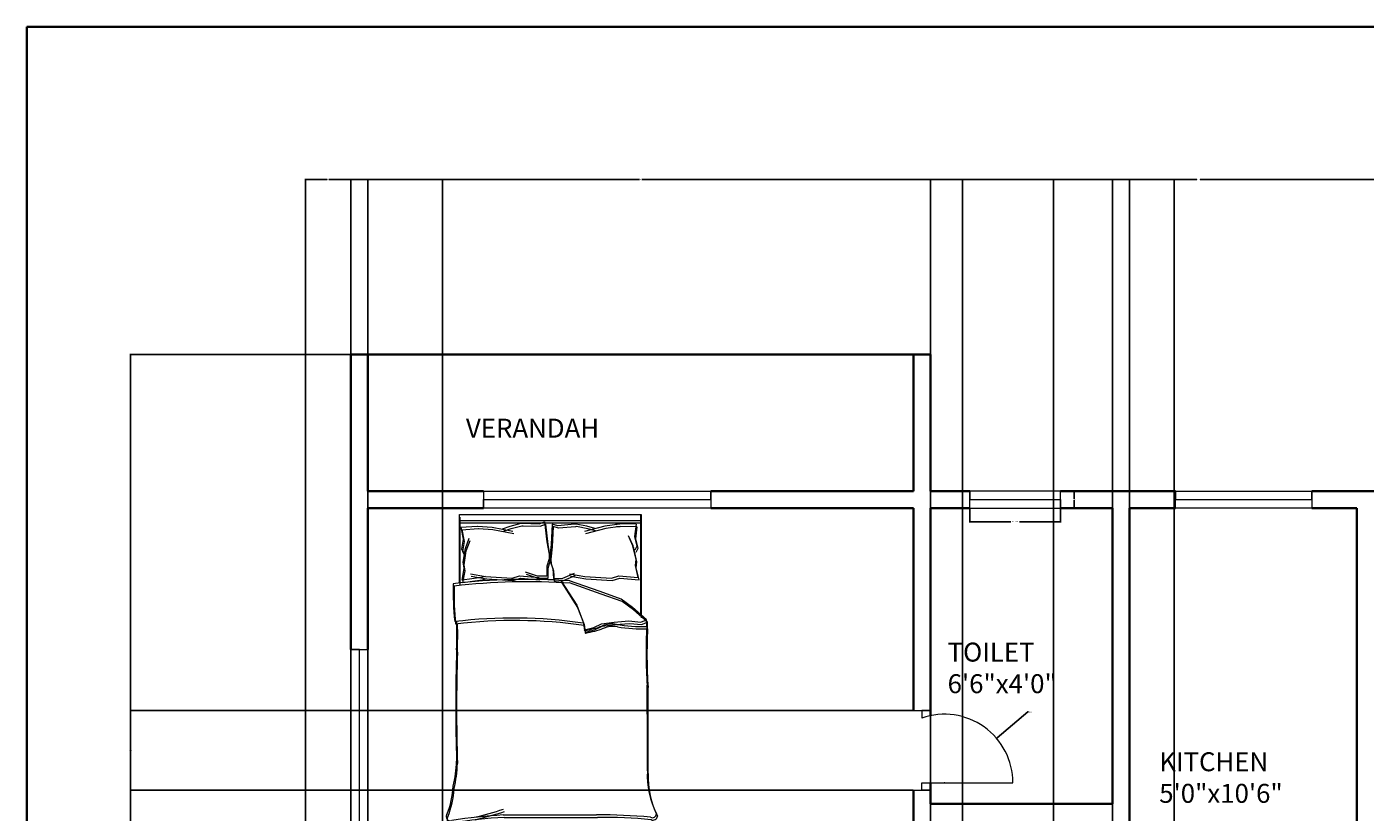
# Model space of a CAD drawing. Units: inches. Extents: x 1937 to 2996, y 1402 to 2323.
# Tile 6 of 10: x 1937 to 2290, y 2116 to 2323. Entities that reach past the tile are written whole.
import ezdxf

# ---------------------------------------------------------------- set-up
doc = ezdxf.new("R2010")
doc.units = ezdxf.units.IN
for name, color, linetype, lineweight in [('A-ANNO-DIMS', 2, 'Continuous', 18), ('A-ANNO-TTLB', 7, 'Continuous', 35), ('A-AREA-IDEN', 7, 'Continuous', 18), ('A-DOOR', 11, 'Continuous', 18), ('A-FURN', 8, 'Continuous', 13), ('A-GLAZ', 141, 'Continuous', 18), ('A-WALL', 7, 'Continuous', 35)]:
    doc.layers.add(name, color=color, linetype=linetype, lineweight=lineweight)
doc.styles.get("Standard").update_dxf_attribs({"font": 'arial.ttf'})
doc.dimstyles.get("Standard").update_dxf_attribs({"dimtxt": 0.18, "dimasz": 0.18, "dimexe": 0.18, "dimexo": 0.0625, "dimgap": 0.09, "dimtad": 0, "dimtih": 1, "dimtoh": 1, "dimdec": 4, "dimzin": 0, "dimdsep": 46, "dimtxsty": 'Standard', "dimcen": 0.09, "dimadec": 0, "dimazin": 0, "dimtfac": 1, "dimtdec": 4, "dimtofl": 0, "dimtmove": 0, "dimatfit": 3, "dimfxl": 1, "dimtolj": 1, "dimtzin": 0, "dimarcsym": 0})

# ---------------------------------------------------------------- blocks, each defined once
blk = doc.blocks.new('BED-DOUBLE')
for p, q in [((-24.01, -18.11), (-24.01, 0)), ((-24.01, -18.11), (-24.01, 0)), ((-24.01, 0), (24.01, 0)), ((23.78, 0), (23.78, -26.61)), ((23.78, 0), (23.78, -26.61)), ((24.01, 0), (24.01, -0.64)), ((-24.01, -1.53), (23.78, -1.53)), ((-24.01, -1.53), (23.78, -1.53)), ((-23.78, -18.75), (-23.78, -0.64)), ((-23.78, -18.75), (-23.78, -0.64)), ((-23.78, -2.17), (24.01, -2.17)), ((-23.78, -2.17), (24.01, -2.17)), ((-23.59, -3.34), (-19.3, -3.01)), ((-23.59, -3.34), (-19.31, -3.01)), ((-23.59, -3.32), (-23.01, -6.5)), ((-23.59, -3.32), (-23.01, -6.5)), ((-19.31, -3.01), (-19.2, -3.03)), ((-19.3, -3.01), (-19.2, -3.03)), ((-19.2, -3.03), (-15.38, -3.32)), ((-19.2, -3.03), (-15.38, -3.32)), ((-15.38, -3.32), (-9.88, -4.33)), ((-15.38, -3.32), (-9.88, -4.33)), ((-12.63, -3.75), (-10.61, -3.03)), ((-12.63, -3.75), (-10.61, -3.03)), ((-10.61, -3.03), (-7.71, -2.3)), ((-10.61, -3.03), (-7.71, -2.3)), ((-10.38, -3.67), (-7.49, -2.94)), ((-10.38, -3.67), (-7.49, -2.94)), ((-7.71, -2.3), (-7.39, -2.3)), ((-7.71, -2.3), (-7.39, -2.3)), ((-7.49, -2.94), (-7.16, -2.94)), ((-7.49, -2.94), (-7.16, -2.94)), ((-7.39, -2.3), (-2.95, -2.45)), ((-7.39, -2.3), (-2.95, -2.45)), ((-7.16, -2.94), (-2.72, -3.09)), ((-7.16, -2.94), (-2.72, -3.09)), ((-2.95, -2.45), (-1.5, -1.87)), ((-2.95, -2.45), (-1.5, -1.87)), ((-2.72, -3.09), (-1.27, -2.51)), ((-2.72, -3.09), (-1.27, -2.51)), ((-1.5, -1.87), (-0.92, -7.22)), ((-1.5, -1.87), (-0.92, -7.22)), ((-1.27, -2.51), (-0.7, -7.86)), ((-1.27, -2.51), (-0.7, -7.86)), ((0.49, -2.49), (0.25, -7.87)), ((0.49, -2.49), (0.25, -7.87)), ((0.72, -3.13), (0.48, -8.51)), ((0.72, -3.13), (0.48, -8.51)), ((1.97, -2.98), (0.49, -2.49)), ((1.97, -2.98), (0.49, -2.49)), ((2.2, -3.62), (0.72, -3.13)), ((2.2, -3.62), (0.72, -3.13)), ((6.4, -2.56), (1.97, -2.98)), ((6.4, -2.56), (1.97, -2.98)), ((6.63, -3.2), (2.2, -3.62)), ((6.63, -3.2), (2.2, -3.62)), ((6.72, -2.54), (6.4, -2.56)), ((6.72, -2.54), (6.4, -2.56)), ((6.95, -3.18), (6.63, -3.2)), ((6.95, -3.18), (6.63, -3.2)), ((9.65, -3.08), (6.72, -2.54)), ((9.65, -3.08), (6.72, -2.54)), ((9.88, -3.72), (6.95, -3.18)), ((9.88, -3.72), (6.95, -3.18)), ((14.43, -3.07), (9.01, -4.42)), ((14.43, -3.07), (9.01, -4.42)), ((11.72, -3.67), (9.65, -3.08)), ((11.72, -3.67), (9.65, -3.08)), ((18.23, -2.54), (14.43, -3.07)), ((18.23, -2.54), (14.43, -3.07)), ((18.46, -3.18), (14.66, -3.71)), ((18.46, -3.18), (14.66, -3.71)), ((22.63, -2.56), (17.23, -2.46)), ((17.23, -2.46), (18.23, -2.54)), ((22.63, -2.56), (17.23, -2.46)), ((17.23, -2.46), (18.23, -2.54)), ((22.86, -3.2), (17.45, -3.1)), ((17.45, -3.1), (18.46, -3.18)), ((22.86, -3.2), (17.45, -3.1)), ((17.45, -3.1), (18.46, -3.18)), ((22.63, -2.56), (22.25, -5.77)), ((22.63, -2.56), (22.25, -5.77)), ((22.86, -3.2), (22.48, -6.41)), ((22.86, -3.2), (22.48, -6.41)), ((24.01, -0.64), (24.01, -27.25)), ((24.01, -0.64), (24.01, -27.25)), ((-23.01, -6.5), (-23.45, -9.1)), ((-23.01, -6.5), (-23.45, -9.1)), ((-23.36, -3.98), (-19.08, -3.65)), ((-23.36, -3.98), (-19.08, -3.65)), ((-23.36, -3.96), (-22.78, -7.14)), ((-23.36, -3.96), (-22.78, -7.14)), ((-22.43, -8.96), (-21.42, -6.21)), ((-22.43, -8.96), (-21.42, -6.21)), ((-22.21, -9.59), (-21.19, -6.85)), ((-22.2, -9.59), (-21.19, -6.85)), ((-19.08, -3.65), (-18.97, -3.67)), ((-19.08, -3.65), (-18.97, -3.67)), ((-18.97, -3.67), (-15.15, -3.96)), ((-18.97, -3.67), (-15.15, -3.96)), ((-15.15, -3.96), (-9.65, -4.97)), ((-15.15, -3.96), (-9.65, -4.97)), ((-12.4, -4.39), (-10.38, -3.67)), ((-12.4, -4.39), (-10.38, -3.67)), ((14.66, -3.71), (9.24, -5.06)), ((14.66, -3.71), (9.24, -5.06)), ((11.94, -4.31), (9.88, -3.72)), ((11.94, -4.31), (9.88, -3.72)), ((21.83, -8.26), (20.64, -5.58)), ((21.82, -8.26), (20.64, -5.58)), ((22.05, -8.9), (20.87, -6.22)), ((22.05, -8.9), (20.87, -6.22)), ((22.25, -5.77), (22.84, -8.34)), ((22.25, -5.77), (22.84, -8.34)), ((22.48, -6.41), (23.07, -8.98)), ((22.48, -6.41), (23.07, -8.98)), ((-23.45, -9.1), (-22.87, -10.11)), ((-23.45, -9.1), (-22.87, -10.11)), ((-22.78, -7.14), (-23.22, -9.74)), ((-22.78, -7.14), (-23.22, -9.74)), ((-23.22, -9.74), (-22.64, -10.75)), ((-23.22, -9.74), (-22.64, -10.75)), ((-23.01, -12.57), (-22.43, -8.96)), ((-23.01, -12.57), (-22.43, -8.96)), ((-22.78, -13.21), (-22.2, -9.59)), ((-22.78, -13.21), (-22.21, -9.59)), ((-0.92, -7.22), (-0.35, -10.4)), ((-0.92, -7.22), (-0.35, -10.4)), ((-0.7, -7.86), (-0.12, -11.04)), ((-0.7, -7.86), (-0.12, -11.04)), ((-0.35, -10.4), (-0.35, -11.7)), ((-0.35, -10.4), (-0.35, -11.7)), ((0.25, -7.87), (-0.13, -11.08)), ((0.25, -7.87), (-0.13, -11.08)), ((0.48, -8.51), (0.1, -11.72)), ((0.48, -8.51), (0.1, -11.72)), ((22.63, -11.83), (21.82, -8.26)), ((22.63, -11.83), (21.83, -8.26)), ((22.86, -12.47), (22.05, -8.9)), ((22.86, -12.47), (22.05, -8.9)), ((22.84, -8.34), (22.33, -9.38)), ((22.84, -8.34), (22.33, -9.38)), ((23.07, -8.98), (22.56, -10.02)), ((23.07, -8.98), (22.56, -10.02)), ((-22.72, -14.16), (-23.01, -12.57)), ((-22.72, -14.16), (-23.01, -12.57)), ((-22.49, -14.8), (-22.78, -13.21)), ((-22.49, -14.8), (-22.78, -13.21)), ((-0.35, -11.7), (-0.92, -13.58)), ((-0.35, -11.7), (-0.92, -13.58)), ((-0.92, -13.58), (-0.92, -16.26)), ((-0.92, -13.58), (-0.92, -16.26)), ((-0.12, -12.34), (-0.7, -14.22)), ((-0.12, -12.34), (-0.7, -14.22)), ((-0.13, -11.08), (-0.05, -12.38)), ((-0.13, -11.08), (-0.05, -12.38)), ((-0.12, -11.04), (-0.12, -12.34)), ((-0.12, -11.04), (-0.12, -12.34)), ((-0.05, -12.38), (0.65, -14.22)), ((-0.05, -12.38), (0.65, -14.22)), ((0.1, -11.72), (0.18, -13.02)), ((0.1, -11.72), (0.18, -13.02)), ((0.18, -13.02), (0.87, -14.86)), ((0.18, -13.02), (0.87, -14.86)), ((22.44, -13.43), (22.63, -11.83)), ((22.44, -13.43), (22.63, -11.83)), ((23.21, -16.57), (22.44, -13.43)), ((23.21, -16.57), (22.44, -13.43)), ((22.67, -14.07), (22.86, -12.47)), ((22.67, -14.07), (22.86, -12.47)), ((23.44, -17.21), (22.67, -14.07)), ((23.44, -17.21), (22.67, -14.07)), ((-23.3, -17.34), (-22.72, -14.16)), ((-23.3, -17.34), (-22.72, -14.16)), ((-18.2, -16.62), (-23.3, -17.34)), ((-18.2, -16.62), (-23.3, -17.34)), ((-23.07, -17.98), (-22.49, -14.8)), ((-23.07, -17.98), (-22.49, -14.8)), ((-17.98, -17.26), (-23.07, -17.98)), ((-17.98, -17.26), (-23.07, -17.98)), ((-21.1, -15.63), (-17.07, -16.3)), ((-21.1, -15.63), (-17.07, -16.3)), ((-20.87, -16.27), (-16.84, -16.93)), ((-20.87, -16.27), (-16.84, -16.93)), ((-17.07, -16.3), (-18.2, -16.62)), ((-17.07, -16.3), (-18.2, -16.62)), ((-16.84, -16.93), (-17.98, -17.26)), ((-16.84, -16.93), (-17.98, -17.26)), ((-17.07, -16.3), (-10.06, -16.73)), ((-17.07, -16.3), (-10.06, -16.73)), ((-16.84, -16.93), (-9.83, -17.37)), ((-16.84, -16.93), (-9.83, -17.37)), ((-10.06, -16.73), (-8.1, -16.17)), ((-10.06, -16.73), (-8.1, -16.17)), ((-9.83, -17.37), (-7.87, -16.81)), ((-9.83, -17.37), (-7.87, -16.81)), ((-8.1, -16.17), (-2.97, -16.57)), ((-8.1, -16.17), (-2.97, -16.57)), ((-7.87, -16.81), (-2.74, -17.21)), ((-7.87, -16.81), (-2.74, -17.21)), ((-3.38, -16.26), (-6.53, -15.17)), ((-3.38, -16.26), (-6.53, -15.17)), ((-3.15, -16.9), (-6.3, -15.81)), ((-3.15, -16.9), (-6.3, -15.81)), ((-0.92, -16.26), (-3.38, -16.26)), ((-0.92, -16.26), (-3.38, -16.26)), ((-0.7, -16.9), (-3.15, -16.9)), ((-0.7, -16.9), (-3.15, -16.9)), ((-0.7, -14.22), (-0.7, -16.9)), ((-0.7, -14.22), (-0.7, -16.9)), ((0.65, -14.22), (0.81, -16.89)), ((0.65, -14.22), (0.81, -16.89)), ((0.81, -16.89), (3.27, -16.74)), ((0.81, -16.89), (3.27, -16.74)), ((0.87, -14.86), (1.04, -17.53)), ((0.87, -14.86), (1.04, -17.53)), ((1.04, -17.53), (3.49, -17.38)), ((1.04, -17.53), (3.49, -17.38)), ((2.77, -17.38), (6.97, -23.88)), ((2.77, -17.38), (6.96, -23.88)), ((3.27, -16.74), (6.34, -15.45)), ((3.27, -16.74), (6.34, -15.45)), ((3.49, -17.38), (6.56, -16.09)), ((3.49, -17.38), (6.56, -16.09)), ((13.16, -20.32), (4.82, -17.38)), ((13.16, -20.32), (4.82, -17.38)), ((5.08, -15.63), (9.11, -16.3)), ((5.08, -15.63), (9.11, -16.3)), ((5.31, -16.27), (9.34, -16.93)), ((5.31, -16.27), (9.34, -16.93)), ((9.11, -16.3), (16.12, -16.73)), ((9.11, -16.3), (16.12, -16.73)), ((9.34, -16.93), (16.35, -17.37)), ((9.34, -16.93), (16.35, -17.37)), ((16.12, -16.73), (18.08, -16.17)), ((16.12, -16.73), (18.08, -16.17)), ((16.35, -17.37), (18.31, -16.81)), ((16.35, -17.37), (18.31, -16.81)), ((18.08, -16.17), (23.21, -16.57)), ((18.08, -16.17), (23.21, -16.57)), ((18.31, -16.81), (23.44, -17.21)), ((18.31, -16.81), (23.44, -17.21)), ((3, -18.02), (7.19, -24.52)), ((3, -18.02), (7.19, -24.52)), ((13.39, -20.96), (5.05, -18.02)), ((13.39, -20.96), (5.05, -18.02)), ((18.74, -22.33), (13.16, -20.32)), ((18.74, -22.33), (13.16, -20.32)), ((18.96, -22.97), (13.39, -20.96)), ((18.96, -22.97), (13.39, -20.96)), ((6.96, -23.88), (8.67, -28.37)), ((6.97, -23.88), (8.67, -28.37)), ((7.19, -24.52), (8.9, -29)), ((7.19, -24.52), (8.9, -29)), ((21.68, -24.5), (18.74, -22.33)), ((21.68, -24.5), (18.74, -22.33)), ((21.91, -25.13), (18.96, -22.97)), ((21.91, -25.13), (18.96, -22.97)), ((25.38, -27.75), (21.68, -24.5)), ((25.38, -27.75), (21.68, -24.5)), ((16.88, -28.37), (20.75, -28.06)), ((16.88, -28.37), (20.75, -28.06)), ((20.75, -28.06), (23.85, -28.37)), ((20.75, -28.06), (23.85, -28.37)), ((25.61, -28.39), (21.91, -25.13)), ((25.61, -28.39), (21.91, -25.13)), ((23.85, -28.37), (25.38, -27.75)), ((23.85, -28.37), (25.38, -27.75)), ((25.46, -29.49), (25.38, -27.75, 3.87)), ((25.46, -29.49), (25.38, -27.75, 3.87)), ((8.67, -28.37), (8.98, -30.38)), ((8.67, -28.37), (8.98, -30.38)), ((8.9, -29), (9.21, -31.02)), ((8.9, -29), (9.21, -31.02)), ((8.98, -30.38), (11.46, -29.76)), ((8.98, -30.38), (11.46, -29.76)), ((9.21, -31.02), (11.68, -30.4)), ((9.21, -31.02), (11.68, -30.4)), ((11.46, -29.76), (13.47, -28.83)), ((11.46, -29.76), (13.47, -28.83)), ((11.68, -30.4), (13.7, -29.47)), ((11.68, -30.4), (13.7, -29.47)), ((13.47, -28.83), (16.88, -28.37)), ((13.47, -28.83), (16.88, -28.37)), ((13.7, -29.47), (17.11, -29)), ((13.7, -29.47), (17.1, -29)), ((17.1, -29), (20.98, -28.69)), ((17.11, -29), (20.98, -28.69)), ((20.98, -28.69), (24.07, -29)), ((20.98, -28.69), (24.07, -29)), ((24.07, -29), (25.61, -28.39)), ((24.07, -29), (25.61, -28.39)), ((25.69, -30.13), (25.61, -28.39, 3.87)), ((25.69, -30.13), (25.61, -28.39, 3.87)), ((-12.42, -79.25), (12.19, -79.25)), ((-12.42, -79.25), (12.19, -79.25)), ((-12.19, -79.88), (12.42, -79.88)), ((-12.19, -79.88), (12.42, -79.88))]:
    blk.add_line(p, q)
for centre, radius, start, end in [((-6.13, -182.05), 164.97, 86.0865, 96.7821), ((-6.13, -182.05), 164.97, 86.0865, 96.7821), ((57.68, -20.1), 83.31, 178.7218, 185.604), ((57.68, -20.1), 83.31, 178.7218, 185.604), ((57.91, -20.74), 83.31, 178.7218, 185.604), ((57.91, -20.74), 83.31, 178.7218, 185.604), ((-5.9, -182.69), 164.97, 86.0865, 96.7821), ((-5.9, -182.69), 164.97, 86.0865, 96.7821), ((-9.73, -156.32), 129.02, 81.7845, 96.9006), ((-9.73, -156.32), 129.02, 81.7845, 96.9006), ((-9.5, -156.96), 129.02, 81.7845, 96.9006), ((-9.5, -156.96), 129.02, 81.7845, 96.9006), ((-194.79, -31.17), 170.11, 358.4762, 1.0082), ((-194.79, -31.17), 170.11, 358.4762, 1.0082), ((-194.56, -31.81), 170.11, 358.4762, 1.0082), ((-194.56, -31.81), 170.11, 358.4762, 1.0082), ((9.15, -30.44), 0.185, 160.2464, 271.1377), ((9.15, -30.44), 0.185, 160.2464, 271.1377), ((3.67, -1.48), 29.65, 280.6617, 289.8806), ((3.67, -1.48), 29.65, 280.6617, 289.8806), ((9.38, -31.08), 0.185, 160.2464, 271.1377), ((9.38, -31.08), 0.185, 160.2464, 271.1377), ((3.9, -2.12), 29.65, 280.6617, 289.8806), ((3.9, -2.12), 29.65, 280.6617, 289.8806), ((16.26, -35.07), 6.22, 78.6608, 113.7384), ((16.26, -35.07), 6.22, 78.6608, 113.7384), ((16.49, -35.71), 6.22, 78.6608, 113.7384), ((16.49, -35.71), 6.22, 78.6608, 113.7384), ((23.84, 6.66), 36.18, 259.8763, 272.5657), ((23.84, 6.66), 36.18, 259.8763, 272.5657), ((24.07, 6.02), 36.18, 259.8763, 272.5657), ((24.07, 6.02), 36.18, 259.8763, 272.5657), ((154.78, -36.32), 129.5, 176.9791, 183.8365), ((154.78, -36.32), 129.5, 176.9791, 183.8365), ((155.01, -36.95), 129.5, 176.9791, 183.8365), ((155.01, -36.95), 129.5, 176.9791, 183.8365), ((457.34, -50.61), 482.31, 178.2277, 181.7185), ((457.34, -50.61), 482.31, 178.2277, 181.7185), ((457.57, -51.25), 482.31, 178.2277, 181.7185), ((457.57, -51.25), 482.31, 178.2277, 181.7185), ((-4536.23, -67.82), 4561.86, 0.00217, 0.28689), ((-4536.23, -67.82), 4561.86, 0.00217, 0.28689), ((-4536, -68.46), 4561.86, 0.00217, 0.28689), ((-4536, -68.46), 4561.86, 0.00217, 0.28689), ((-54.38, -64.52), 29.63, 346.0648, 358.9113), ((-54.38, -64.52), 29.63, 346.0648, 358.9113), ((-54.16, -65.15), 29.63, 346.0648, 358.9113), ((-54.16, -65.15), 29.63, 346.0648, 358.9113), ((48.67, -68.67), 23.07, 177.4714, 206.4681), ((48.67, -68.67), 23.07, 177.4714, 206.4681), ((48.9, -69.31), 23.07, 177.4714, 206.4681), ((48.9, -69.31), 23.07, 177.4714, 206.4681), ((-49.14, -70.28), 23.56, 337.9751, 356.652), ((-49.14, -70.28), 23.56, 337.9751, 356.652), ((-48.92, -70.91), 23.56, 337.9751, 356.652), ((-48.92, -70.91), 23.56, 337.9751, 356.652), ((-44.71, 23.71), 106.46, 283.3832, 287.7053), ((-44.71, 23.71), 106.46, 283.3832, 287.7053), ((-26.4, -79.72), 1.09, 146.1736, 293.4781), ((-26.4, -79.72), 1.09, 146.1736, 293.4781), ((-26.17, -80.36), 1.09, 146.1736, 293.4781), ((-26.17, -80.36), 1.09, 146.1736, 293.4781), ((-6.06, -200.84), 121.76, 92.9958, 99.4091), ((-6.06, -200.84), 121.76, 92.9958, 99.4091), ((-5.83, -201.48), 121.76, 92.9958, 99.4091), ((-5.83, -201.48), 121.76, 92.9958, 99.4091), ((-44.48, 23.07), 106.46, 283.3832, 287.7053), ((-44.48, 23.07), 106.46, 283.3832, 287.7053), ((13.67, -212.28), 133.04, 84.4998, 90.6351), ((13.67, -212.28), 133.04, 84.4998, 90.6351), ((13.9, -212.92), 133.04, 84.4998, 90.6351), ((13.9, -212.92), 133.04, 84.4998, 90.6351), ((26.93, -78.87), 1.1, 242.6588, 356.02), ((26.93, -78.87), 1.1, 242.6588, 356.02), ((27.15, -79.51), 1.1, 242.6588, 356.02), ((27.15, -79.51), 1.1, 242.6588, 356.02)]:
    blk.add_arc(centre, radius, start, end)
blk = doc.blocks.new('WINDOW-60IN')
for p, q in [((0, 2.25), (0, -2.25)), ((0, 2.25), (60, 2.25)), ((0, -2.25), (0, 0)), ((0, 0), (60, 0)), ((60, 0), (60, 2.25)), ((60, 2.25), (60, -2.25)), ((60, -2.25), (0, -2.25))]:
    blk.add_line(p, q)
blk = doc.blocks.new('WINDOW-24IN')
for p, q in [((0, -2.25), (0, 2.25)), ((0, 2.25), (0, 0)), ((24, 2.25), (0, 2.25)), ((0, 0), (24, 0)), ((24, -2.25), (24, 2.25)), ((24, 0), (24, -2.25)), ((0, -2.25), (24, -2.25))]:
    blk.add_line(p, q)
blk = doc.blocks.new('*D13')
at = {"layer": 'A-ANNO-DIMS', "color": 0, "lineweight": -2, "transparency": 16777216}
for p, q in [((2185.99, 2196.24), (2185.99, 2192.53)), ((2209.99, 2196.24), (2209.99, 2192.53)), ((2186.17, 2192.71), (2196.87, 2192.71)), ((2209.81, 2192.71), (2199.11, 2192.71))]:
    blk.add_line(p, q, dxfattribs=at)
at = {"layer": 'A-ANNO-DIMS', "color": 0, "transparency": 16777216}
for points in [[(2186.17, 2192.74), (2186.17, 2192.68), (2185.99, 2192.71)], [(2209.81, 2192.74), (2209.81, 2192.68), (2209.99, 2192.71)]]:
    blk.add_solid(points, dxfattribs=at)
at = {"layer": 'Defpoints', "color": 0, "transparency": 16777216}
for p in [(2185.99, 2196.31), (2209.99, 2196.31), (2209.99, 2192.71)]:
    blk.add_point(p, dxfattribs=at)
at = {"layer": 'A-ANNO-DIMS', "color": 0, "transparency": 16777216, "insert": (2197.99, 2192.71), "char_height": 0.18, "attachment_point": 5}
blk.add_mtext('\\A1;WINDOW 24 TYP.', dxfattribs=at)
blk = doc.blocks.new('*D14')
at = {"layer": 'A-ANNO-DIMS', "color": 0, "lineweight": -2, "transparency": 16777216}
for p, q in [((2210.06, 2200.81), (2213.77, 2200.81)), ((2213.59, 2200.63), (2213.59, 2198.74)), ((2213.59, 2196.49), (2213.59, 2198.37)), ((2210.06, 2196.31), (2213.77, 2196.31))]:
    blk.add_line(p, q, dxfattribs=at)
at = {"layer": 'A-ANNO-DIMS', "color": 0, "transparency": 16777216}
for points in [[(2213.56, 2200.63), (2213.62, 2200.63), (2213.59, 2200.81)], [(2213.56, 2196.49), (2213.62, 2196.49), (2213.59, 2196.31)]]:
    blk.add_solid(points, dxfattribs=at)
at = {"layer": 'Defpoints', "color": 0, "transparency": 16777216}
for p in [(2209.99, 2200.81), (2213.59, 2200.81), (2209.99, 2196.31)]:
    blk.add_point(p, dxfattribs=at)
at = {"layer": 'A-ANNO-DIMS', "color": 0, "transparency": 16777216, "insert": (2213.59, 2198.56), "char_height": 0.18, "attachment_point": 5}
blk.add_mtext('\\A1;5 TYP.', dxfattribs=at)
blk = doc.blocks.new('*D24')
at = {"layer": 'A-ANNO-DIMS', "color": 0, "lineweight": -2, "transparency": 16777216}
for p, q in [((2022.58, 2236.81), (1964.32, 2236.81)), ((1964.5, 2236.63), (1964.5, 1896.24)), ((1964.5, 1555.49), (1964.5, 1895.87)), ((2022.58, 1555.31), (1964.32, 1555.31))]:
    blk.add_line(p, q, dxfattribs=at)
at = {"layer": 'A-ANNO-DIMS', "color": 0, "transparency": 16777216}
for points in [[(1964.47, 2236.63), (1964.53, 2236.63), (1964.5, 2236.81)], [(1964.47, 1555.49), (1964.53, 1555.49), (1964.5, 1555.31)]]:
    blk.add_solid(points, dxfattribs=at)
at = {"layer": 'Defpoints', "color": 0, "transparency": 16777216}
for p in [(1964.5, 2236.81), (2022.65, 2236.81), (2022.65, 1555.31)]:
    blk.add_point(p, dxfattribs=at)
at = {"layer": 'A-ANNO-DIMS', "color": 0, "transparency": 16777216, "insert": (1964.5, 1896.06), "char_height": 0.18, "attachment_point": 5}
blk.add_mtext('\\A1;681.5', dxfattribs=at)
blk = doc.blocks.new('*D25')
at = {"layer": 'A-ANNO-DIMS', "color": 0, "lineweight": -2, "transparency": 16777216}
for p, q in [((2022.65, 2236.87), (2022.65, 2283.14)), ((2022.83, 2282.96), (2098.87, 2282.96)), ((2175.47, 2282.96), (2099.43, 2282.96)), ((2175.65, 2236.87), (2175.65, 2283.14))]:
    blk.add_line(p, q, dxfattribs=at)
at = {"layer": 'A-ANNO-DIMS', "color": 0, "transparency": 16777216}
for points in [[(2022.83, 2282.99), (2022.83, 2282.93), (2022.65, 2282.96)], [(2175.47, 2282.99), (2175.47, 2282.93), (2175.65, 2282.96)]]:
    blk.add_solid(points, dxfattribs=at)
at = {"layer": 'Defpoints', "color": 0, "transparency": 16777216}
for p in [(2175.65, 2282.96), (2022.65, 2236.81), (2175.65, 2236.81)]:
    blk.add_point(p, dxfattribs=at)
at = {"layer": 'A-ANNO-DIMS', "color": 0, "transparency": 16777216, "insert": (2099.15, 2282.96), "char_height": 0.18, "attachment_point": 5}
blk.add_mtext('\\A1;153', dxfattribs=at)
blk = doc.blocks.new('*D26')
at = {"layer": 'A-ANNO-DIMS', "color": 0, "lineweight": -2, "transparency": 16777216}
for p, q in [((2175.65, 2236.87), (2175.65, 2283.14)), ((2175.83, 2282.96), (2245.91, 2282.96)), ((2316.9, 2282.96), (2246.82, 2282.96)), ((2317.08, 2236.87), (2317.08, 2283.14))]:
    blk.add_line(p, q, dxfattribs=at)
at = {"layer": 'A-ANNO-DIMS', "color": 0, "transparency": 16777216}
for points in [[(2175.83, 2282.99), (2175.83, 2282.93), (2175.65, 2282.96)], [(2316.9, 2282.99), (2316.9, 2282.93), (2317.08, 2282.96)]]:
    blk.add_solid(points, dxfattribs=at)
at = {"layer": 'Defpoints', "color": 0, "transparency": 16777216}
for p in [(2317.08, 2282.96), (2175.65, 2236.81), (2317.08, 2236.81)]:
    blk.add_point(p, dxfattribs=at)
at = {"layer": 'A-ANNO-DIMS', "color": 0, "transparency": 16777216, "insert": (2246.36, 2282.96), "char_height": 0.18, "attachment_point": 5}
blk.add_mtext('\\A1;141.43', dxfattribs=at)
blk = doc.blocks.new('*D44')
at = {"layer": 'A-ANNO-DIMS', "color": 0, "lineweight": -2, "transparency": 16777216}
for p, q in [((2010.65, 1769.37), (2010.65, 2283.14)), ((2010.83, 2282.96), (2016.44, 2282.96)), ((2022.47, 2282.96), (2016.86, 2282.96)), ((2022.65, 1769.37), (2022.65, 2283.14))]:
    blk.add_line(p, q, dxfattribs=at)
at = {"layer": 'A-ANNO-DIMS', "color": 0, "transparency": 16777216}
for points in [[(2010.83, 2282.99), (2010.83, 2282.93), (2010.65, 2282.96)], [(2022.47, 2282.99), (2022.47, 2282.93), (2022.65, 2282.96)]]:
    blk.add_solid(points, dxfattribs=at)
at = {"layer": 'Defpoints', "color": 0, "transparency": 16777216}
for p in [(2022.65, 2282.96), (2010.65, 1769.31), (2022.65, 1769.31)]:
    blk.add_point(p, dxfattribs=at)
at = {"layer": 'A-ANNO-DIMS', "color": 0, "transparency": 16777216, "insert": (2016.65, 2282.96), "char_height": 0.18, "attachment_point": 5}
blk.add_mtext('\\A1;12', dxfattribs=at)
blk = doc.blocks.new('*D46')
at = {"layer": 'A-ANNO-DIMS', "color": 0, "lineweight": -2, "transparency": 16777216}
for p, q in [((2027.15, 1591.37), (2027.15, 2283.14)), ((2027.33, 2282.96), (2036.53, 2282.96)), ((2046.64, 2282.96), (2037.44, 2282.96)), ((2046.82, 1591.37), (2046.82, 2283.14))]:
    blk.add_line(p, q, dxfattribs=at)
at = {"layer": 'A-ANNO-DIMS', "color": 0, "transparency": 16777216}
for points in [[(2027.33, 2282.99), (2027.33, 2282.93), (2027.15, 2282.96)], [(2046.64, 2282.99), (2046.64, 2282.93), (2046.82, 2282.96)]]:
    blk.add_solid(points, dxfattribs=at)
at = {"layer": 'Defpoints', "color": 0, "transparency": 16777216}
for p in [(2046.82, 2282.96), (2027.15, 1591.31), (2046.82, 1591.31)]:
    blk.add_point(p, dxfattribs=at)
at = {"layer": 'A-ANNO-DIMS', "color": 0, "transparency": 16777216, "insert": (2036.99, 2282.96), "char_height": 0.18, "attachment_point": 5}
blk.add_mtext('\\A1;19.678', dxfattribs=at)
blk = doc.blocks.new('*D47')
at = {"layer": 'A-ANNO-DIMS', "color": 0, "lineweight": -2, "transparency": 16777216}
for p, q in [((2175.65, 1591.37), (2175.65, 2283.14)), ((2175.83, 2282.96), (2179.52, 2282.96)), ((2183.96, 2282.96), (2180.27, 2282.96)), ((2184.14, 1591.37), (2184.14, 2283.14))]:
    blk.add_line(p, q, dxfattribs=at)
at = {"layer": 'A-ANNO-DIMS', "color": 0, "transparency": 16777216}
for points in [[(2175.83, 2282.99), (2175.83, 2282.93), (2175.65, 2282.96)], [(2183.96, 2282.99), (2183.96, 2282.93), (2184.14, 2282.96)]]:
    blk.add_solid(points, dxfattribs=at)
at = {"layer": 'Defpoints', "color": 0, "transparency": 16777216}
for p in [(2184.14, 2282.96), (2175.65, 1591.31), (2184.14, 1591.31)]:
    blk.add_point(p, dxfattribs=at)
at = {"layer": 'A-ANNO-DIMS', "color": 0, "transparency": 16777216, "insert": (2179.89, 2282.96), "char_height": 0.18, "attachment_point": 5}
blk.add_mtext('\\A1;8.491', dxfattribs=at)
blk = doc.blocks.new('*D48')
at = {"layer": 'A-ANNO-DIMS', "color": 0, "lineweight": -2, "transparency": 16777216}
for p, q in [((2208.14, 1591.37), (2208.14, 2283.14)), ((2208.32, 2282.96), (2223.66, 2282.96)), ((2239.78, 2282.96), (2224.44, 2282.96)), ((2239.96, 1591.37), (2239.96, 2283.14))]:
    blk.add_line(p, q, dxfattribs=at)
at = {"layer": 'A-ANNO-DIMS', "color": 0, "transparency": 16777216}
for points in [[(2208.32, 2282.99), (2208.32, 2282.93), (2208.14, 2282.96)], [(2239.78, 2282.99), (2239.78, 2282.93), (2239.96, 2282.96)]]:
    blk.add_solid(points, dxfattribs=at)
at = {"layer": 'Defpoints', "color": 0, "transparency": 16777216}
for p in [(2239.96, 2282.96), (2208.14, 1591.31), (2239.96, 1591.31)]:
    blk.add_point(p, dxfattribs=at)
at = {"layer": 'A-ANNO-DIMS', "color": 0, "transparency": 16777216, "insert": (2224.05, 2282.96), "char_height": 0.18, "attachment_point": 5}
blk.add_mtext('\\A1;31.82', dxfattribs=at)
blk = doc.blocks.new('*D49')
at = {"layer": 'A-ANNO-DIMS', "color": 0, "lineweight": -2, "transparency": 16777216}
for p, q in [((2223.65, 2095.03), (2223.65, 2283.14)), ((2223.83, 2282.96), (2225.64, 2282.96)), ((2227.97, 2282.96), (2226.16, 2282.96)), ((2228.15, 2095.03), (2228.15, 2283.14))]:
    blk.add_line(p, q, dxfattribs=at)
at = {"layer": 'A-ANNO-DIMS', "color": 0, "transparency": 16777216}
for points in [[(2223.83, 2282.99), (2223.83, 2282.93), (2223.65, 2282.96)], [(2227.97, 2282.99), (2227.97, 2282.93), (2228.15, 2282.96)]]:
    blk.add_solid(points, dxfattribs=at)
at = {"layer": 'Defpoints', "color": 0, "transparency": 16777216}
for p in [(2228.15, 2282.96), (2223.65, 2094.97), (2228.15, 2094.97)]:
    blk.add_point(p, dxfattribs=at)
at = {"layer": 'A-ANNO-DIMS', "color": 0, "transparency": 16777216, "insert": (2225.9, 2282.96), "char_height": 0.18, "attachment_point": 5}
blk.add_mtext('\\A1;4.5', dxfattribs=at)
blk = doc.blocks.new('*D53')
at = {"layer": 'A-ANNO-DIMS', "color": 0, "lineweight": -2, "transparency": 16777216}
for p, q in [((2171.08, 2142.9), (1964.32, 2142.9)), ((1964.5, 2142.72), (1964.5, 2132.56)), ((1964.5, 2122.03), (1964.5, 2132.19)), ((2171.08, 2121.85), (1964.32, 2121.85))]:
    blk.add_line(p, q, dxfattribs=at)
at = {"layer": 'A-ANNO-DIMS', "color": 0, "transparency": 16777216}
for points in [[(1964.47, 2142.72), (1964.53, 2142.72), (1964.5, 2142.9)], [(1964.47, 2122.03), (1964.53, 2122.03), (1964.5, 2121.85)]]:
    blk.add_solid(points, dxfattribs=at)
at = {"layer": 'Defpoints', "color": 0, "transparency": 16777216}
for p in [(1964.5, 2142.9), (2171.15, 2142.9), (2171.15, 2121.85)]:
    blk.add_point(p, dxfattribs=at)
at = {"layer": 'A-ANNO-DIMS', "color": 0, "transparency": 16777216, "insert": (1964.5, 2132.38), "char_height": 0.18, "attachment_point": 5}
blk.add_mtext('\\A1;21.054', dxfattribs=at)
blk = doc.blocks.new('*D73')
at = {"layer": 'A-ANNO-DIMS', "color": 0, "lineweight": -2, "transparency": 16777216}
for p, q in [((2201.38, 2142.53), (2193.25, 2135.64)), ((2201.56, 2142.53), (2201.38, 2142.53)), ((2179.25, 2123.85), (2179.43, 2123.85)), ((2179.34, 2123.76), (2179.34, 2123.94))]:
    blk.add_line(p, q, dxfattribs=at)
at = {"layer": 'A-ANNO-DIMS', "color": 0, "transparency": 16777216}
blk.add_solid([(2193.24, 2135.66), (2193.27, 2135.62), (2193.12, 2135.52)], dxfattribs=at)
at = {"layer": 'Defpoints', "color": 0, "transparency": 16777216}
for p in [(2193.12, 2135.52), (2179.34, 2123.85)]:
    blk.add_point(p, dxfattribs=at)
at = {"layer": 'A-ANNO-DIMS', "color": 0, "transparency": 16777216, "insert": (2202.04, 2142.53), "char_height": 0.18, "attachment_point": 5}
blk.add_mtext('\\A1;R18.06', dxfattribs=at)

msp = doc.modelspace()

# ---------------------------------------------------------------- linework, layer by layer
at = {"layer": 'A-ANNO-TTLB'}
msp.add_lwpolyline([(1937.1125, 2323.2883), (2995.8132, 2323.2883), (2995.8132, 1401.6335), (1937.1125, 1401.6335)], close=True, dxfattribs=at)
at = {"layer": 'A-DOOR'}
for p, q in [((2171.1473, 2142.9035), (2175.6473, 2142.9035)), ((2175.6473, 2142.9035), (2173.3973, 2142.9035)), ((2173.3973, 2142.9035), (2173.3973, 2140.9035)), ((2173.3973, 2121.8495), (2173.3973, 2123.8495)), ((2173.3973, 2123.8495), (2197.3973, 2123.8495)), ((2171.1473, 2121.8495), (2175.6473, 2121.8495)), ((2175.6473, 2121.8495), (2173.3973, 2121.8495))]:
    msp.add_line(p, q, dxfattribs=at)
msp.add_arc((2179.3382, 2123.8495), 18.0591, 360, 109.206044, dxfattribs=at)
at = {"layer": 'A-GLAZ'}
for p, q in [((2240.3117, 2196.3061), (2240.3117, 2200.8061)), ((2240.3117, 2200.8061), (2240.3117, 2198.5561)), ((2240.3117, 2200.8061), (2276.3117, 2200.8061)), ((2240.3117, 2198.5561), (2276.3117, 2198.5561)), ((2276.3117, 2198.5561), (2276.3117, 2200.8061)), ((2276.3117, 2200.8061), (2276.3117, 2196.3061)), ((2276.3117, 2196.3061), (2240.3117, 2196.3061))]:
    msp.add_line(p, q, dxfattribs=at)
at = {"layer": 'A-WALL'}
for p, q in [((2022.6473, 2200.8061), (2022.6473, 2236.8061)), ((2022.6473, 2236.8061), (2175.6473, 2236.8061)), ((2027.1473, 2200.8061), (2027.1473, 2236.8061)), ((2171.1473, 2200.8061), (2171.1473, 2236.8061)), ((2175.6473, 2236.8061), (2175.6473, 2200.8061)), ((2022.6473, 2200.8061), (2022.6473, 2159.0049)), ((2027.1473, 2200.8061), (2057.6392, 2200.8061)), ((2117.6392, 2200.8061), (2171.1473, 2200.8061)), ((2175.6473, 2200.8061), (2185.9926, 2200.8061)), ((2209.9926, 2200.8061), (2240.3117, 2200.8061)), ((2276.3117, 2200.8061), (2317.081, 2200.8061)), ((2027.1473, 2196.3061), (2057.6392, 2196.3061)), ((2027.1473, 2196.3061), (2027.1473, 2159.0049)), ((2117.6392, 2196.3061), (2171.1473, 2196.3061)), ((2171.1473, 2196.3061), (2171.1473, 2142.9035)), ((2175.6473, 2196.3061), (2175.6473, 2141.5275)), ((2175.6473, 2196.3061), (2185.9926, 2196.3061)), ((2209.9926, 2196.3061), (2223.6473, 2196.3061)), ((2223.6473, 2196.3061), (2223.6473, 2118.3061)), ((2228.1473, 2196.3061), (2228.1473, 2093.5364)), ((2228.1473, 2196.3061), (2240.3117, 2196.3061)), ((2276.3117, 2196.3061), (2288.1473, 2196.3061)), ((2288.1473, 2196.3061), (2288.1473, 2070.3061)), ((2175.6473, 2123.8495), (2175.6473, 2118.3061)), ((2171.1473, 2121.8495), (2171.1473, 2103.4818)), ((2175.6473, 2118.3061), (2223.6473, 2118.3061))]:
    msp.add_line(p, q, dxfattribs=at)

# ---------------------------------------------------------------- block references
at = {"layer": 'A-FURN'}
msp.add_blockref('BED-DOUBLE', (2075.3048, 2194.5807), dxfattribs=at)
at = {"layer": 'A-GLAZ'}
for name, p in [('WINDOW-60IN', (2057.6392, 2198.5561)), ('WINDOW-24IN', (2185.9926, 2198.5561))]:
    msp.add_blockref(name, p, dxfattribs=at)
at = {"layer": 'A-GLAZ', "rotation": 90}
msp.add_blockref('WINDOW-60IN', (2024.8973, 2099.0049), dxfattribs=at)

# ---------------------------------------------------------------- texts
at = {"layer": 'A-AREA-IDEN', "char_height": 5, "attachment_point": 1}
for s, width, insert in [('VERANDAH', 137.071433, (2053.0327, 2219.8875)), ('TOILET\\P6\'6"x4\'0"', 136.477078, (2180.1702, 2160.7998)), ('KITCHEN\\P5\'0"x10\'6"', 122.863889, (2236.0229, 2131.8684))]:
    msp.add_mtext_dynamic_manual_height_columns(s, width=width, gutter_width=12.5, heights=[0], dxfattribs=dict(at, insert=insert))

# ---------------------------------------------------------------- dimensions: what is measured, and where the dimension line sits
at = {"layer": 'A-ANNO-DIMS'}
for base, p1, p2, override, picture, middle in [((2022.6473, 2282.9561), (2010.6473, 1769.3061), (2022.6473, 1769.3061), {"dimdec": 0, "dimlfac": 1, "dimrnd": 0, "dimzin": 0, "dimdsep": 46, "dimlunit": 2}, '*D44', (2016.6473, 2282.9561)), ((2175.6473, 2282.9561), (2022.6473, 2236.8061), (2175.6473, 2236.8061), {"dimdec": 0, "dimlfac": 1, "dimrnd": 0, "dimzin": 0, "dimdsep": 46, "dimlunit": 2}, '*D25', (2099.1473, 2282.9561)), ((2046.82483, 2282.95612), (2027.14731, 1591.30612), (2046.82483, 1591.30612), {"dimdec": 3, "dimlfac": 1, "dimrnd": 0, "dimzin": 0, "dimdsep": 46, "dimlunit": 2}, '*D46', (2036.98607, 2282.95612)), ((2317.081, 2282.9561), (2175.6473, 2236.8061), (2317.081, 2236.8061), {"dimdec": 2, "dimlfac": 1, "dimrnd": 0, "dimzin": 0, "dimdsep": 46, "dimlunit": 2}, '*D26', (2246.3642, 2282.9561)), ((2184.1385, 2282.9561), (2175.6473, 1591.3061), (2184.1385, 1591.3061), {"dimdec": 3, "dimlfac": 1, "dimrnd": 0, "dimzin": 0, "dimdsep": 46, "dimlunit": 2}, '*D47', (2179.8929, 2282.9561)), ((2239.9586, 2282.9561), (2208.1385, 1591.3061), (2239.9586, 1591.3061), {"dimdec": 2, "dimlfac": 1, "dimrnd": 0, "dimzin": 0, "dimdsep": 46, "dimlunit": 2}, '*D48', (2224.0486, 2282.9561)), ((2228.1473, 2282.9561), (2223.6473, 2094.9699), (2228.1473, 2094.9699), {"dimdec": 1, "dimlfac": 1, "dimrnd": 0, "dimzin": 0, "dimdsep": 46, "dimlunit": 2}, '*D49', (2225.8973, 2282.9561))]:
    dim = msp.add_linear_dim(base=base, p1=p1, p2=p2, dimstyle='Standard', override=override, dxfattribs=at)
    dim.commit()
    dim.dimension.update_dxf_attribs({"geometry": picture, "text_midpoint": middle})
for base, p1, p2, override, picture, middle in [((1964.4973, 2236.8061), (2022.6473, 1555.3061), (2022.6473, 2236.8061), {"dimdec": 1, "dimlfac": 1, "dimrnd": 0, "dimzin": 0, "dimdsep": 46, "dimlunit": 2}, '*D24', (1964.4973, 1896.0561)), ((1964.4973, 2142.9035), (2171.1473, 2121.8495), (2171.1473, 2142.9035), {"dimdec": 3, "dimlfac": 1, "dimrnd": 0, "dimzin": 0, "dimdsep": 46, "dimlunit": 2}, '*D53', (1964.4973, 2132.3765))]:
    dim = msp.add_linear_dim(base=base, p1=p1, p2=p2, angle=90, dimstyle='Standard', override=override, dxfattribs=at)
    dim.commit()
    dim.dimension.update_dxf_attribs({"geometry": picture, "text_midpoint": middle})
dim = msp.add_linear_dim(base=(2213.5925526002, 2200.8061190364), p1=(2209.9925526002, 2196.3061190364), p2=(2209.9925526002, 2200.8061190364), angle=90, text='<> TYP.', dimstyle='Standard', override={"dimdec": 0, "dimlfac": 1, "dimrnd": 0, "dimzin": 0, "dimdsep": 46, "dimlunit": 2}, dxfattribs=at)
dim.commit()
dim.dimension.update_dxf_attribs({"geometry": '*D14', "text_midpoint": (2213.5925526002, 2198.5561190364)})
dim = msp.add_linear_dim(base=(2209.9926, 2192.7061), p1=(2185.9926, 2196.3061), p2=(2209.9926, 2196.3061), text='WINDOW <> TYP.', dimstyle='Standard', override={"dimdec": 0, "dimlfac": 1, "dimrnd": 0, "dimzin": 0, "dimdsep": 46, "dimlunit": 2}, dxfattribs=at)
dim.commit()
dim.dimension.update_dxf_attribs({"geometry": '*D13', "text_midpoint": (2197.9926, 2192.7061)})
dim = msp.add_radius_dim(center=(2179.3382, 2123.8495), mpoint=(2193.1173, 2135.5229), dimstyle='Standard', override={"dimdec": 2, "dimlfac": 1, "dimrnd": 0, "dimzin": 0, "dimdsep": 46, "dimlunit": 2}, dxfattribs=at)
dim.commit()
dim.dimension.update_dxf_attribs({"geometry": '*D73', "text_midpoint": (2202.0445, 2142.527), "dimtype": 164})

doc.saveas('drawing.dxf')
